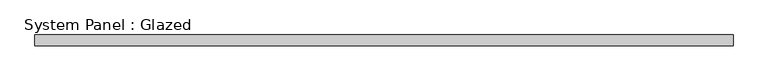
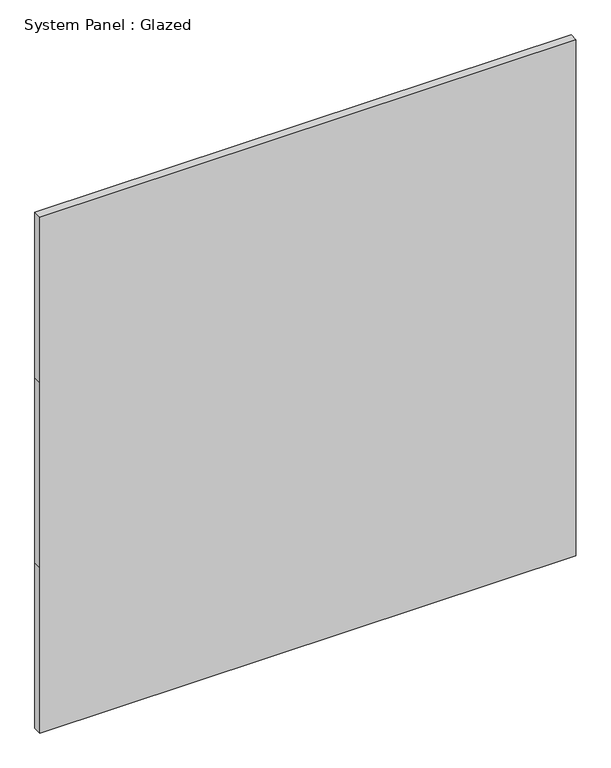
"""IFC4 building model written with IfcOpenShell, lengths in millimetres: plate geometry, System Panel : Glazed."""

from ifc_helpers import new_model, si_unit, frame, origin, place, context, project, spatial, polyline, outline, extrude, source, transform, mapped, element, save


def system_panel_glazed_35d8d551(model_context):
    return source(origin(), model_context, "Body", "SweptSolid", [
        extrude(outline(polyline([(0.0, -815.975), (0.0, 815.975), (532.0236621, 815.975), (1127.5473242, 815.975), (1659.5709863, 815.975), (1659.5709863, -815.975), (1127.5473242, -815.975), (532.0236621, -815.975), (0.0, -815.975)])), frame((0.0, 19.05, 0.0), z_axis=(0.0, 1.0, 0.0), x_axis=(0.0, 0.0, 1.0)), (0.0, 0.0, 1.0), 25.4),
    ])


if __name__ == "__main__":
    model = new_model("IFC4")
    model_context = context("Model", 3, world=origin())
    ifc_project = project(units=[si_unit("LENGTHUNIT", "METRE", prefix="MILLI")], contexts=[model_context])
    site = spatial("IfcSite", under=ifc_project)
    building = spatial("IfcBuilding", under=site)
    placement = place(None, origin())
    system_panel_glazed_shape = system_panel_glazed_35d8d551(model_context)
    element("IfcPlate", 1, ObjectType="System Panel : Glazed", at=placement, inside=building, context=model_context, shape_type="MappedRepresentation", body=[
        mapped(system_panel_glazed_shape, transform((0.0, 0.0, 0.0), x_axis=(1.0, 0.0, 0.0), y_axis=(0.0, 1.0, 0.0), z_axis=(0.0, 0.0, 1.0))),
    ])
    save(model, "model.ifc")

# Revit data of these elements
# Type "System Panel : Glazed"
#   Construction Type Id = "GSP4R"
#   Analytic Construction = "1/8 in Pilkington single glazing"
#   Visual Light Transmittance = 0.9
#   Solar Heat Gain Coefficient = 0.86
#   Heat Transfer Coefficient (U) = 1.18115 BTU/(h·ft²·°F)
#   Define Thermal Properties by = 1
# Element 1 (IfcPlate, "System Panel : Glazed")
#   Materials on its faces: "Glass"
# Materials
#   "Glass": class "Glass", colour RGB 0 128 192, transparency 0.75, Description = "Soda Lime Glass", Cost = 0
